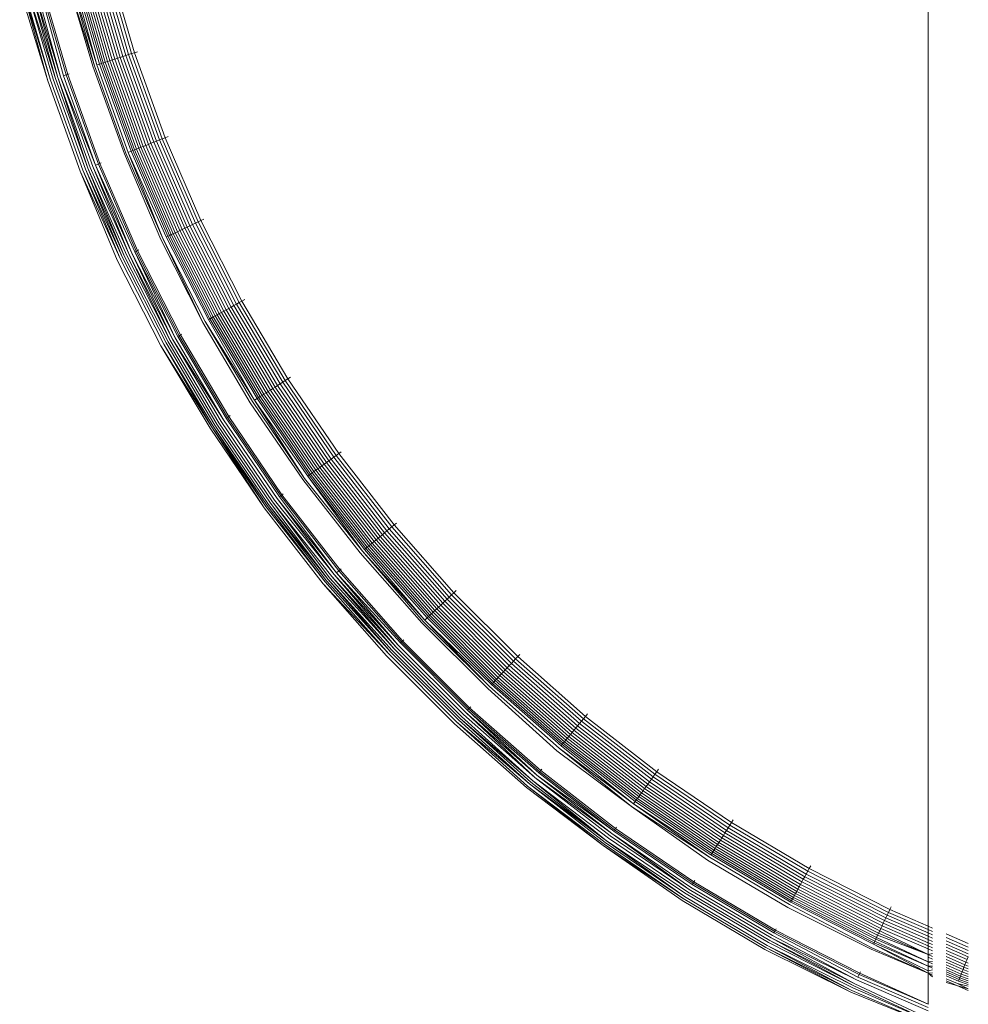
# Model space of a CAD drawing. Units: inches. Extents: x 64 to 1167, y 117 to 939.
# Tile 42 of 56: x 1129.1618 to 1129.8616, y 499.9133 to 500.6393. Entities that reach past the tile are written whole.
import ezdxf

# ---------------------------------------------------------------- set-up
doc = ezdxf.new("R2010")
doc.units = ezdxf.units.IN
doc.header["$MEASUREMENT"] = 0
doc.layers.add('A-FLOR-FIXT', color=8, linetype='Continuous', lineweight=18)

msp = doc.modelspace()

# ---------------------------------------------------------------- linework, layer by layer
at = {"layer": 'A-FLOR-FIXT'}
for p, q in [((1129.83185, 499.97088), (1129.83185, 500.69852)), ((1129.20936, 500.67419), (1129.22829, 500.60906)), ((1129.21118, 500.67466), (1129.23007, 500.60964)), ((1129.21308, 500.67515), (1129.23194, 500.61024)), ((1129.21505, 500.67566), (1129.23387, 500.61087)), ((1129.21709, 500.67618), (1129.23587, 500.61152)), ((1129.21918, 500.67672), (1129.23793, 500.61219)), ((1129.22132, 500.67727), (1129.24003, 500.61288)), ((1129.2235, 500.67783), (1129.24217, 500.61357)), ((1129.22571, 500.67839), (1129.24434, 500.61427)), ((1129.22794, 500.67896), (1129.24652, 500.61498)), ((1129.19606, 500.67078), (1129.21694, 500.60537)), ((1129.19606, 500.67078), (1129.2158, 500.605)), ((1129.19859, 500.67143), (1129.21862, 500.60592)), ((1129.19859, 500.67143), (1129.21694, 500.60537)), ((1129.20057, 500.67194), (1129.21862, 500.60592)), ((1129.20175, 500.67224), (1129.22081, 500.60663)), ((1129.20305, 500.67257), (1129.22209, 500.60705)), ((1129.20447, 500.67294), (1129.22348, 500.6075)), ((1129.206, 500.67333), (1129.22498, 500.60799)), ((1129.20763, 500.67375), (1129.22659, 500.60851)), ((1129.16182, 500.66199), (1129.1825, 500.59418)), ((1129.16358, 500.66244), (1129.1825, 500.59418)), ((1129.16358, 500.66244), (1129.18443, 500.59481)), ((1129.1647, 500.66273), (1129.18443, 500.59481)), ((1129.16683, 500.66327), (1129.18817, 500.59602)), ((1129.16683, 500.66327), (1129.18652, 500.59549)), ((1129.16942, 500.66394), (1129.19, 500.59662)), ((1129.16942, 500.66394), (1129.18817, 500.59602)), ((1129.17135, 500.66444), (1129.19197, 500.59726)), ((1129.17135, 500.66444), (1129.19, 500.59662)), ((1129.17342, 500.66497), (1129.19197, 500.59726)), ((1129.17558, 500.66552), (1129.19404, 500.59793)), ((1129.17668, 500.6658), (1129.1962, 500.59863)), ((1129.1778, 500.66609), (1129.19729, 500.59899)), ((1129.22829, 500.60906), (1129.22659, 500.60851)), ((1129.23007, 500.60964), (1129.22829, 500.60906)), ((1129.22829, 500.60906), (1129.25126, 500.54524)), ((1129.23194, 500.61024), (1129.23007, 500.60964)), ((1129.23007, 500.60964), (1129.25301, 500.54593)), ((1129.23387, 500.61087), (1129.23194, 500.61024)), ((1129.23194, 500.61024), (1129.25483, 500.54665)), ((1129.23587, 500.61152), (1129.23387, 500.61087)), ((1129.23387, 500.61087), (1129.25672, 500.5474)), ((1129.23793, 500.61219), (1129.23587, 500.61152)), ((1129.23587, 500.61152), (1129.25868, 500.54818)), ((1129.24003, 500.61288), (1129.23793, 500.61219)), ((1129.23793, 500.61219), (1129.26069, 500.54897)), ((1129.24217, 500.61357), (1129.24003, 500.61288)), ((1129.24003, 500.61288), (1129.26274, 500.54979)), ((1129.24434, 500.61427), (1129.24217, 500.61357)), ((1129.24217, 500.61357), (1129.26484, 500.55061)), ((1129.24652, 500.61498), (1129.24434, 500.61427)), ((1129.24434, 500.61427), (1129.26695, 500.55145)), ((1129.24872, 500.6157), (1129.24652, 500.61498)), ((1129.24652, 500.61498), (1129.26909, 500.5523)), ((1129.2158, 500.605), (1129.23905, 500.54041)), ((1129.21694, 500.60537), (1129.24017, 500.54085)), ((1129.22081, 500.60663), (1129.21862, 500.60592)), ((1129.21862, 500.60592), (1129.24181, 500.5415)), ((1129.22209, 500.60705), (1129.22081, 500.60663)), ((1129.22081, 500.60663), (1129.24395, 500.54235)), ((1129.22348, 500.6075), (1129.22209, 500.60705)), ((1129.22209, 500.60705), (1129.2452, 500.54284)), ((1129.22498, 500.60799), (1129.22348, 500.6075)), ((1129.22348, 500.6075), (1129.24657, 500.54338)), ((1129.22659, 500.60851), (1129.22498, 500.60799)), ((1129.22498, 500.60799), (1129.24803, 500.54396)), ((1129.22659, 500.60851), (1129.2496, 500.54458)), ((1129.18443, 500.59481), (1129.20839, 500.52827)), ((1129.18652, 500.59549), (1129.21043, 500.52907)), ((1129.18817, 500.59602), (1129.21205, 500.52971)), ((1129.19, 500.59662), (1129.21383, 500.53042)), ((1129.19, 500.59662), (1129.21205, 500.52971)), ((1129.19197, 500.59726), (1129.21575, 500.53118)), ((1129.19197, 500.59726), (1129.21779, 500.53199)), ((1129.1962, 500.59863), (1129.19404, 500.59793)), ((1129.19404, 500.59793), (1129.21779, 500.53199)), ((1129.19729, 500.59899), (1129.1962, 500.59863)), ((1129.1962, 500.59863), (1129.21989, 500.53282)), ((1129.19839, 500.59934), (1129.19729, 500.59899)), ((1129.19729, 500.59899), (1129.22096, 500.53324)), ((1129.1825, 500.59418), (1129.2065, 500.52752)), ((1129.26695, 500.55145), (1129.26484, 500.55061)), ((1129.26909, 500.5523), (1129.26695, 500.55145)), ((1129.26695, 500.55145), (1129.29347, 500.49018)), ((1129.27124, 500.55315), (1129.26909, 500.5523)), ((1129.26909, 500.5523), (1129.29555, 500.49115)), ((1129.2452, 500.54284), (1129.24657, 500.54338)), ((1129.24657, 500.54338), (1129.24803, 500.54396)), ((1129.24657, 500.54338), (1129.27363, 500.48084)), ((1129.24803, 500.54396), (1129.2496, 500.54458)), ((1129.24803, 500.54396), (1129.27506, 500.48151)), ((1129.2496, 500.54458), (1129.25126, 500.54524)), ((1129.2496, 500.54458), (1129.27658, 500.48223)), ((1129.25126, 500.54524), (1129.25301, 500.54593)), ((1129.25126, 500.54524), (1129.2782, 500.48299)), ((1129.25483, 500.54665), (1129.25301, 500.54593)), ((1129.25301, 500.54593), (1129.2799, 500.48379)), ((1129.25672, 500.5474), (1129.25483, 500.54665)), ((1129.25483, 500.54665), (1129.28167, 500.48462)), ((1129.25868, 500.54818), (1129.25672, 500.5474)), ((1129.25672, 500.5474), (1129.28352, 500.48549)), ((1129.26069, 500.54897), (1129.25868, 500.54818)), ((1129.25868, 500.54818), (1129.28542, 500.48639)), ((1129.26274, 500.54979), (1129.26069, 500.54897)), ((1129.26069, 500.54897), (1129.28738, 500.48731)), ((1129.26484, 500.55061), (1129.26274, 500.54979)), ((1129.26274, 500.54979), (1129.28937, 500.48825)), ((1129.26484, 500.55061), (1129.29141, 500.48921)), ((1129.23905, 500.54041), (1129.26598, 500.47724)), ((1129.24017, 500.54085), (1129.2674, 500.47791)), ((1129.24181, 500.5415), (1129.24395, 500.54235)), ((1129.24181, 500.5415), (1129.26998, 500.47912)), ((1129.24181, 500.5415), (1129.2674, 500.47791)), ((1129.24395, 500.54235), (1129.2452, 500.54284)), ((1129.24395, 500.54235), (1129.27109, 500.47964)), ((1129.2452, 500.54284), (1129.27231, 500.48022)), ((1129.21043, 500.52907), (1129.23775, 500.46396)), ((1129.21043, 500.52907), (1129.23923, 500.46465)), ((1129.21205, 500.52971), (1129.24089, 500.46543)), ((1129.21205, 500.52971), (1129.23923, 500.46465)), ((1129.21383, 500.53042), (1129.24269, 500.46628)), ((1129.21575, 500.53118), (1129.24269, 500.46628)), ((1129.21575, 500.53118), (1129.24462, 500.46719)), ((1129.21989, 500.53282), (1129.21779, 500.53199)), ((1129.21779, 500.53199), (1129.24664, 500.46814)), ((1129.21779, 500.53199), (1129.24462, 500.46719)), ((1129.22096, 500.53324), (1129.21989, 500.53282)), ((1129.21989, 500.53282), (1129.24767, 500.46862)), ((1129.22203, 500.53367), (1129.22096, 500.53324)), ((1129.22096, 500.53324), (1129.24871, 500.46911)), ((1129.2065, 500.52752), (1129.23382, 500.46211)), ((1129.2065, 500.52752), (1129.23593, 500.4631)), ((1129.20839, 500.52827), (1129.23593, 500.4631)), ((1129.20839, 500.52827), (1129.23775, 500.46396)), ((1129.28352, 500.48549), (1129.28167, 500.48462)), ((1129.28542, 500.48639), (1129.28352, 500.48549)), ((1129.28352, 500.48549), (1129.31414, 500.42538)), ((1129.28738, 500.48731), (1129.28542, 500.48639)), ((1129.28542, 500.48639), (1129.31599, 500.4264)), ((1129.28937, 500.48825), (1129.28738, 500.48731)), ((1129.28738, 500.48731), (1129.31788, 500.42744)), ((1129.29141, 500.48921), (1129.28937, 500.48825)), ((1129.28937, 500.48825), (1129.31982, 500.4285)), ((1129.29347, 500.49018), (1129.29141, 500.48921)), ((1129.29141, 500.48921), (1129.32179, 500.42959)), ((1129.29555, 500.49115), (1129.29347, 500.49018)), ((1129.29347, 500.49018), (1129.32378, 500.43068)), ((1129.29764, 500.49214), (1129.29555, 500.49115)), ((1129.29555, 500.49115), (1129.3258, 500.43179)), ((1129.27109, 500.47964), (1129.26998, 500.47912)), ((1129.26998, 500.47912), (1129.30104, 500.41818)), ((1129.27231, 500.48022), (1129.27109, 500.47964)), ((1129.27109, 500.47964), (1129.30211, 500.41877)), ((1129.27363, 500.48084), (1129.27231, 500.48022)), ((1129.27231, 500.48022), (1129.30328, 500.41941)), ((1129.27506, 500.48151), (1129.27363, 500.48084)), ((1129.27363, 500.48084), (1129.30457, 500.42012)), ((1129.27658, 500.48223), (1129.27506, 500.48151)), ((1129.27506, 500.48151), (1129.30595, 500.42088)), ((1129.2782, 500.48299), (1129.27658, 500.48223)), ((1129.27658, 500.48223), (1129.30743, 500.42169)), ((1129.2799, 500.48379), (1129.2782, 500.48299)), ((1129.2782, 500.48299), (1129.30899, 500.42255)), ((1129.28167, 500.48462), (1129.2799, 500.48379)), ((1129.2799, 500.48379), (1129.31064, 500.42346)), ((1129.28167, 500.48462), (1129.31236, 500.4244)), ((1129.26598, 500.47724), (1129.29696, 500.41594)), ((1129.2674, 500.47791), (1129.29854, 500.4168)), ((1129.2674, 500.47791), (1129.29696, 500.41594)), ((1129.23775, 500.46396), (1129.26982, 500.40102)), ((1129.23923, 500.46465), (1129.27125, 500.4018)), ((1129.24089, 500.46543), (1129.27285, 500.40269)), ((1129.24269, 500.46628), (1129.27461, 500.40365)), ((1129.24269, 500.46628), (1129.27285, 500.40269)), ((1129.24462, 500.46719), (1129.27648, 500.40468)), ((1129.24462, 500.46719), (1129.27461, 500.40365)), ((1129.24664, 500.46814), (1129.24767, 500.46862)), ((1129.24664, 500.46814), (1129.27843, 500.40575)), ((1129.24664, 500.46814), (1129.27648, 500.40468)), ((1129.24767, 500.46862), (1129.24871, 500.46911)), ((1129.24767, 500.46862), (1129.27943, 500.4063)), ((1129.24871, 500.46911), (1129.24976, 500.4696)), ((1129.24871, 500.46911), (1129.28043, 500.40685)), ((1129.23382, 500.46211), (1129.26602, 500.39893)), ((1129.23593, 500.4631), (1129.26805, 500.40005)), ((1129.31788, 500.42744), (1129.31599, 500.4264)), ((1129.31982, 500.4285), (1129.31788, 500.42744)), ((1129.31788, 500.42744), (1129.35208, 500.3696)), ((1129.32179, 500.42959), (1129.31982, 500.4285)), ((1129.31982, 500.4285), (1129.35395, 500.37079)), ((1129.32378, 500.43068), (1129.32179, 500.42959)), ((1129.32179, 500.42959), (1129.35585, 500.37199)), ((1129.3258, 500.43179), (1129.32378, 500.43068)), ((1129.32378, 500.43068), (1129.35777, 500.37321)), ((1129.32782, 500.4329), (1129.3258, 500.43179)), ((1129.3258, 500.43179), (1129.35971, 500.37445)), ((1129.30457, 500.42012), (1129.30328, 500.41941)), ((1129.30595, 500.42088), (1129.30457, 500.42012)), ((1129.30457, 500.42012), (1129.33926, 500.36146)), ((1129.30743, 500.42169), (1129.30595, 500.42088)), ((1129.30595, 500.42088), (1129.34059, 500.36231)), ((1129.30899, 500.42255), (1129.30743, 500.42169)), ((1129.30743, 500.42169), (1129.34201, 500.36321)), ((1129.31064, 500.42346), (1129.30899, 500.42255)), ((1129.30899, 500.42255), (1129.34352, 500.36417)), ((1129.31236, 500.4244), (1129.31064, 500.42346)), ((1129.31064, 500.42346), (1129.34511, 500.36518)), ((1129.31414, 500.42538), (1129.31236, 500.4244)), ((1129.31236, 500.4244), (1129.34676, 500.36623)), ((1129.31599, 500.4264), (1129.31414, 500.42538)), ((1129.31414, 500.42538), (1129.34848, 500.36732)), ((1129.31599, 500.4264), (1129.35026, 500.36845)), ((1129.29696, 500.41594), (1129.33193, 500.35681)), ((1129.29854, 500.4168), (1129.33494, 500.35872)), ((1129.29854, 500.4168), (1129.33344, 500.35778)), ((1129.30211, 500.41877), (1129.30104, 500.41818)), ((1129.30104, 500.41818), (1129.33494, 500.35872)), ((1129.30328, 500.41941), (1129.30211, 500.41877)), ((1129.30211, 500.41877), (1129.33689, 500.35996)), ((1129.30328, 500.41941), (1129.33802, 500.36068)), ((1129.27943, 500.4063), (1129.27843, 500.40575)), ((1129.27843, 500.40575), (1129.31407, 500.34548)), ((1129.28043, 500.40685), (1129.27943, 500.4063)), ((1129.27943, 500.4063), (1129.31503, 500.34609)), ((1129.28145, 500.40741), (1129.28043, 500.40685)), ((1129.28043, 500.40685), (1129.316, 500.34671)), ((1129.26602, 500.39893), (1129.30237, 500.33805)), ((1129.26602, 500.39893), (1129.30362, 500.33885)), ((1129.26805, 500.40005), (1129.30459, 500.33946)), ((1129.26805, 500.40005), (1129.30362, 500.33885)), ((1129.26982, 500.40102), (1129.30578, 500.34022)), ((1129.27125, 500.4018), (1129.30716, 500.34109)), ((1129.27285, 500.40269), (1129.3087, 500.34207)), ((1129.27461, 500.40365), (1129.31039, 500.34314)), ((1129.27461, 500.40365), (1129.31219, 500.34429)), ((1129.27648, 500.40468), (1129.31219, 500.34429)), ((1129.35208, 500.3696), (1129.35026, 500.36845)), ((1129.35395, 500.37079), (1129.35208, 500.3696)), ((1129.35208, 500.3696), (1129.38985, 500.31403)), ((1129.35585, 500.37199), (1129.35395, 500.37079)), ((1129.35395, 500.37079), (1129.39164, 500.31533)), ((1129.35777, 500.37321), (1129.35585, 500.37199)), ((1129.35585, 500.37199), (1129.39346, 500.31665)), ((1129.35971, 500.37445), (1129.35777, 500.37321)), ((1129.35777, 500.37321), (1129.3953, 500.31799)), ((1129.36166, 500.37568), (1129.35971, 500.37445)), ((1129.35971, 500.37445), (1129.39716, 500.31934)), ((1129.33926, 500.36146), (1129.34059, 500.36231)), ((1129.34059, 500.36231), (1129.34201, 500.36321)), ((1129.34059, 500.36231), (1129.37884, 500.30603)), ((1129.34201, 500.36321), (1129.34352, 500.36417)), ((1129.34201, 500.36321), (1129.3802, 500.30702)), ((1129.34352, 500.36417), (1129.34511, 500.36518)), ((1129.34352, 500.36417), (1129.38165, 500.30807)), ((1129.34511, 500.36518), (1129.34676, 500.36623)), ((1129.34511, 500.36518), (1129.38317, 500.30917)), ((1129.34848, 500.36732), (1129.34676, 500.36623)), ((1129.34676, 500.36623), (1129.38475, 500.31033)), ((1129.35026, 500.36845), (1129.34848, 500.36732)), ((1129.34848, 500.36732), (1129.3864, 500.31152)), ((1129.35026, 500.36845), (1129.3881, 500.31276)), ((1129.33193, 500.35681), (1129.37072, 500.30013)), ((1129.33344, 500.35778), (1129.37199, 500.30105)), ((1129.33494, 500.35872), (1129.33689, 500.35996)), ((1129.33494, 500.35872), (1129.3743, 500.30273)), ((1129.33494, 500.35872), (1129.37199, 500.30105)), ((1129.33689, 500.35996), (1129.33802, 500.36068)), ((1129.33689, 500.35996), (1129.37529, 500.30345)), ((1129.33802, 500.36068), (1129.33926, 500.36146)), ((1129.33802, 500.36068), (1129.37638, 500.30424)), ((1129.33926, 500.36146), (1129.37756, 500.3051)), ((1129.316, 500.34671), (1129.31698, 500.34733)), ((1129.30578, 500.34022), (1129.34548, 500.28179)), ((1129.30716, 500.34109), (1129.3468, 500.28275)), ((1129.3087, 500.34207), (1129.34828, 500.28383)), ((1129.31039, 500.34314), (1129.3499, 500.285)), ((1129.31219, 500.34429), (1129.35163, 500.28626)), ((1129.31407, 500.34548), (1129.31503, 500.34609)), ((1129.31407, 500.34548), (1129.35343, 500.28757)), ((1129.31503, 500.34609), (1129.316, 500.34671)), ((1129.31503, 500.34609), (1129.35435, 500.28824)), ((1129.316, 500.34671), (1129.35528, 500.28891)), ((1129.30237, 500.33805), (1129.34221, 500.27942)), ((1129.30362, 500.33885), (1129.34341, 500.28029)), ((1129.30362, 500.33885), (1129.34221, 500.27942)), ((1129.30459, 500.33946), (1129.34434, 500.28097)), ((1129.30459, 500.33946), (1129.34341, 500.28029)), ((1129.3953, 500.31799), (1129.39716, 500.31934)), ((1129.39716, 500.31934), (1129.39903, 500.3207)), ((1129.39716, 500.31934), (1129.438, 500.2667)), ((1129.38475, 500.31033), (1129.3864, 500.31152)), ((1129.3864, 500.31152), (1129.3881, 500.31276)), ((1129.3864, 500.31152), (1129.42775, 500.25822)), ((1129.3881, 500.31276), (1129.38985, 500.31403)), ((1129.3881, 500.31276), (1129.42937, 500.25956)), ((1129.38985, 500.31403), (1129.39164, 500.31533)), ((1129.38985, 500.31403), (1129.43103, 500.26094)), ((1129.39164, 500.31533), (1129.39346, 500.31665)), ((1129.39164, 500.31533), (1129.43274, 500.26235)), ((1129.39346, 500.31665), (1129.3953, 500.31799)), ((1129.39346, 500.31665), (1129.43447, 500.26378)), ((1129.3953, 500.31799), (1129.43622, 500.26523)), ((1129.37638, 500.30424), (1129.37529, 500.30345)), ((1129.37756, 500.3051), (1129.37638, 500.30424)), ((1129.37638, 500.30424), (1129.4182, 500.25032)), ((1129.37884, 500.30603), (1129.37756, 500.3051)), ((1129.37756, 500.3051), (1129.41933, 500.25126)), ((1129.3802, 500.30702), (1129.37884, 500.30603)), ((1129.37884, 500.30603), (1129.42055, 500.25226)), ((1129.38165, 500.30807), (1129.3802, 500.30702)), ((1129.3802, 500.30702), (1129.42184, 500.25334)), ((1129.38317, 500.30917), (1129.38165, 500.30807)), ((1129.38165, 500.30807), (1129.42322, 500.25447)), ((1129.38475, 500.31033), (1129.38317, 500.30917)), ((1129.38317, 500.30917), (1129.42467, 500.25567)), ((1129.38475, 500.31033), (1129.42618, 500.25692)), ((1129.37072, 500.30013), (1129.4131, 500.24611)), ((1129.37199, 500.30105), (1129.41465, 500.24739)), ((1129.37529, 500.30345), (1129.3743, 500.30273)), ((1129.3743, 500.30273), (1129.41465, 500.24739)), ((1129.3743, 500.30273), (1129.41622, 500.24869)), ((1129.37529, 500.30345), (1129.41716, 500.24946)), ((1129.35528, 500.28891), (1129.35621, 500.28959)), ((1129.3468, 500.28275), (1129.38938, 500.22648)), ((1129.34828, 500.28383), (1129.3922, 500.22881)), ((1129.34828, 500.28383), (1129.39072, 500.22759)), ((1129.3499, 500.285), (1129.39379, 500.23013)), ((1129.35163, 500.28626), (1129.39548, 500.23152)), ((1129.35163, 500.28626), (1129.39379, 500.23013)), ((1129.35343, 500.28757), (1129.35435, 500.28824)), ((1129.35343, 500.28757), (1129.39548, 500.23152)), ((1129.35435, 500.28824), (1129.35528, 500.28891)), ((1129.35435, 500.28824), (1129.39722, 500.23297)), ((1129.35528, 500.28891), (1129.39811, 500.2337)), ((1129.34221, 500.27942), (1129.38566, 500.2234)), ((1129.34341, 500.28029), (1129.38722, 500.2247)), ((1129.34434, 500.28097), (1129.38722, 500.2247)), ((1129.34548, 500.28179), (1129.38938, 500.22648)), ((1129.34548, 500.28179), (1129.38821, 500.22551)), ((1129.43977, 500.26817), (1129.438, 500.2667)), ((1129.43103, 500.26094), (1129.42937, 500.25956)), ((1129.43274, 500.26235), (1129.43103, 500.26094)), ((1129.43103, 500.26094), (1129.47547, 500.21054)), ((1129.43447, 500.26378), (1129.43274, 500.26235)), ((1129.43274, 500.26235), (1129.47708, 500.21205)), ((1129.43622, 500.26523), (1129.43447, 500.26378)), ((1129.43447, 500.26378), (1129.47872, 500.21359)), ((1129.438, 500.2667), (1129.43622, 500.26523)), ((1129.43622, 500.26523), (1129.48038, 500.21515)), ((1129.438, 500.2667), (1129.48206, 500.21672)), ((1129.42184, 500.25334), (1129.42055, 500.25226)), ((1129.42322, 500.25447), (1129.42184, 500.25334)), ((1129.42184, 500.25334), (1129.46677, 500.20237)), ((1129.42467, 500.25567), (1129.42322, 500.25447)), ((1129.42322, 500.25447), (1129.46808, 500.2036)), ((1129.42618, 500.25692), (1129.42467, 500.25567)), ((1129.42467, 500.25567), (1129.46944, 500.20488)), ((1129.42775, 500.25822), (1129.42618, 500.25692)), ((1129.42618, 500.25692), (1129.47087, 500.20622)), ((1129.42937, 500.25956), (1129.42775, 500.25822)), ((1129.42775, 500.25822), (1129.47236, 500.20762)), ((1129.42937, 500.25956), (1129.47389, 500.20906)), ((1129.4131, 500.24611), (1129.45851, 500.19461)), ((1129.41465, 500.24739), (1129.46066, 500.19663)), ((1129.41465, 500.24739), (1129.45938, 500.19543)), ((1129.41716, 500.24946), (1129.41622, 500.24869)), ((1129.41622, 500.24869), (1129.46066, 500.19663)), ((1129.4182, 500.25032), (1129.41716, 500.24946)), ((1129.41716, 500.24946), (1129.46235, 500.19821)), ((1129.41933, 500.25126), (1129.4182, 500.25032)), ((1129.4182, 500.25032), (1129.46333, 500.19914)), ((1129.42055, 500.25226), (1129.41933, 500.25126)), ((1129.41933, 500.25126), (1129.4644, 500.20014)), ((1129.42055, 500.25226), (1129.46555, 500.20122)), ((1129.39722, 500.23297), (1129.39548, 500.23152)), ((1129.39548, 500.23152), (1129.44265, 500.17972)), ((1129.39548, 500.23152), (1129.44103, 500.17819)), ((1129.39811, 500.2337), (1129.39722, 500.23297)), ((1129.39722, 500.23297), (1129.44348, 500.1805)), ((1129.399, 500.23444), (1129.39811, 500.2337)), ((1129.39811, 500.2337), (1129.44432, 500.18129)), ((1129.38722, 500.2247), (1129.43402, 500.17161)), ((1129.38821, 500.22551), (1129.43549, 500.17299)), ((1129.38938, 500.22648), (1129.43668, 500.17411)), ((1129.38938, 500.22648), (1129.43549, 500.17299)), ((1129.39072, 500.22759), (1129.43801, 500.17536)), ((1129.3922, 500.22881), (1129.43947, 500.17673)), ((1129.3922, 500.22881), (1129.43801, 500.17536)), ((1129.39379, 500.23013), (1129.44103, 500.17819)), ((1129.39379, 500.23013), (1129.43947, 500.17673)), ((1129.38566, 500.2234), (1129.43241, 500.1701)), ((1129.38566, 500.2234), (1129.43402, 500.17161)), ((1129.48206, 500.21672), (1129.48038, 500.21515)), ((1129.48374, 500.2183), (1129.48206, 500.21672)), ((1129.48206, 500.21672), (1129.52917, 500.16961)), ((1129.47547, 500.21054), (1129.47389, 500.20906)), ((1129.47708, 500.21205), (1129.47547, 500.21054)), ((1129.47547, 500.21054), (1129.52298, 500.16302)), ((1129.47872, 500.21359), (1129.47708, 500.21205)), ((1129.47708, 500.21205), (1129.52449, 500.16464)), ((1129.48038, 500.21515), (1129.47872, 500.21359)), ((1129.47872, 500.21359), (1129.52603, 500.16628)), ((1129.48038, 500.21515), (1129.52759, 500.16794)), ((1129.46677, 500.20237), (1129.46555, 500.20122)), ((1129.46808, 500.2036), (1129.46677, 500.20237)), ((1129.46677, 500.20237), (1129.51482, 500.15433)), ((1129.46944, 500.20488), (1129.46808, 500.2036)), ((1129.46808, 500.2036), (1129.51604, 500.15563)), ((1129.47087, 500.20622), (1129.46944, 500.20488)), ((1129.46944, 500.20488), (1129.51732, 500.157)), ((1129.47236, 500.20762), (1129.47087, 500.20622)), ((1129.47087, 500.20622), (1129.51867, 500.15843)), ((1129.47389, 500.20906), (1129.47236, 500.20762)), ((1129.47236, 500.20762), (1129.52006, 500.15992)), ((1129.47389, 500.20906), (1129.5215, 500.16145)), ((1129.45938, 500.19543), (1129.50843, 500.14753)), ((1129.46235, 500.19821), (1129.46066, 500.19663)), ((1129.46066, 500.19663), (1129.50843, 500.14753)), ((1129.46066, 500.19663), (1129.50982, 500.14901)), ((1129.46333, 500.19914), (1129.46235, 500.19821)), ((1129.46235, 500.19821), (1129.51066, 500.1499)), ((1129.4644, 500.20014), (1129.46333, 500.19914)), ((1129.46333, 500.19914), (1129.51158, 500.15088)), ((1129.46555, 500.20122), (1129.4644, 500.20014)), ((1129.4644, 500.20014), (1129.51258, 500.15195)), ((1129.46555, 500.20122), (1129.51366, 500.1531)), ((1129.45851, 500.19461), (1129.50705, 500.14606)), ((1129.44265, 500.17972), (1129.44348, 500.1805)), ((1129.44348, 500.1805), (1129.44432, 500.18129)), ((1129.44348, 500.1805), (1129.49294, 500.13104)), ((1129.44432, 500.18129), (1129.44516, 500.18208)), ((1129.44432, 500.18129), (1129.49373, 500.13188)), ((1129.43668, 500.17411), (1129.48655, 500.12424)), ((1129.43801, 500.17536), (1129.48781, 500.12557)), ((1129.43947, 500.17673), (1129.48918, 500.12703)), ((1129.44103, 500.17819), (1129.49064, 500.12858)), ((1129.44265, 500.17972), (1129.49216, 500.13021)), ((1129.43241, 500.1701), (1129.48254, 500.11996)), ((1129.43402, 500.17161), (1129.48406, 500.12158)), ((1129.43549, 500.17299), (1129.48544, 500.12305)), ((1129.52603, 500.16628), (1129.52449, 500.16464)), ((1129.52759, 500.16794), (1129.52603, 500.16628)), ((1129.52603, 500.16628), (1129.57622, 500.12203)), ((1129.52917, 500.16961), (1129.52759, 500.16794)), ((1129.52759, 500.16794), (1129.57768, 500.12378)), ((1129.53075, 500.17129), (1129.52917, 500.16961)), ((1129.52917, 500.16961), (1129.57914, 500.12555)), ((1129.52006, 500.15992), (1129.51867, 500.15843)), ((1129.5215, 500.16145), (1129.52006, 500.15992)), ((1129.52006, 500.15992), (1129.57066, 500.1153)), ((1129.52298, 500.16302), (1129.5215, 500.16145)), ((1129.5215, 500.16145), (1129.572, 500.11692)), ((1129.52449, 500.16464), (1129.52298, 500.16302)), ((1129.52298, 500.16302), (1129.57338, 500.11859)), ((1129.52449, 500.16464), (1129.57479, 500.12029)), ((1129.51258, 500.15195), (1129.51158, 500.15088)), ((1129.51366, 500.1531), (1129.51258, 500.15195)), ((1129.51258, 500.15195), (1129.5637, 500.10689)), ((1129.51482, 500.15433), (1129.51366, 500.1531)), ((1129.51366, 500.1531), (1129.56471, 500.1081)), ((1129.51604, 500.15563), (1129.51482, 500.15433)), ((1129.51482, 500.15433), (1129.56578, 500.1094)), ((1129.51732, 500.157), (1129.51604, 500.15563)), ((1129.51604, 500.15563), (1129.56692, 500.11078)), ((1129.51867, 500.15843), (1129.51732, 500.157)), ((1129.51732, 500.157), (1129.56811, 500.11222)), ((1129.51867, 500.15843), (1129.56936, 500.11373)), ((1129.50705, 500.14606), (1129.55816, 500.1002)), ((1129.50843, 500.14753), (1129.55983, 500.10221)), ((1129.51066, 500.1499), (1129.50982, 500.14901)), ((1129.50982, 500.14901), (1129.56113, 500.10378)), ((1129.51158, 500.15088), (1129.51066, 500.1499)), ((1129.51066, 500.1499), (1129.56191, 500.10472)), ((1129.51158, 500.15088), (1129.56277, 500.10576)), ((1129.49216, 500.13021), (1129.49294, 500.13104)), ((1129.49216, 500.13021), (1129.54326, 500.08218)), ((1129.49216, 500.13021), (1129.54469, 500.0839)), ((1129.49294, 500.13104), (1129.49373, 500.13188)), ((1129.49294, 500.13104), (1129.54541, 500.08478)), ((1129.49373, 500.13188), (1129.49452, 500.13272)), ((1129.49373, 500.13188), (1129.54614, 500.08567)), ((1129.48544, 500.12305), (1129.53796, 500.07577)), ((1129.48655, 500.12424), (1129.54003, 500.07828)), ((1129.48655, 500.12424), (1129.53893, 500.07694)), ((1129.48781, 500.12557), (1129.54003, 500.07828)), ((1129.48918, 500.12703), (1129.5419, 500.08054)), ((1129.49064, 500.12858), (1129.54326, 500.08218)), ((1129.49064, 500.12858), (1129.5419, 500.08054)), ((1129.57768, 500.12378), (1129.57622, 500.12203)), ((1129.57914, 500.12555), (1129.57768, 500.12378)), ((1129.57768, 500.12378), (1129.63043, 500.08286)), ((1129.58061, 500.12733), (1129.57914, 500.12555)), ((1129.57914, 500.12555), (1129.63178, 500.08472)), ((1129.48254, 500.11996), (1129.53573, 500.07307)), ((1129.48406, 500.12158), (1129.53649, 500.07399)), ((1129.48406, 500.12158), (1129.53796, 500.07577)), ((1129.57066, 500.1153), (1129.56936, 500.11373)), ((1129.572, 500.11692), (1129.57066, 500.1153)), ((1129.57066, 500.1153), (1129.62397, 500.07396)), ((1129.57338, 500.11859), (1129.572, 500.11692)), ((1129.572, 500.11692), (1129.6252, 500.07566)), ((1129.57479, 500.12029), (1129.57338, 500.11859)), ((1129.57338, 500.11859), (1129.62647, 500.07741)), ((1129.57622, 500.12203), (1129.57479, 500.12029)), ((1129.57479, 500.12029), (1129.62777, 500.0792)), ((1129.57622, 500.12203), (1129.62909, 500.08101)), ((1129.56471, 500.1081), (1129.5637, 500.10689)), ((1129.56578, 500.1094), (1129.56471, 500.1081)), ((1129.56471, 500.1081), (1129.61847, 500.0664)), ((1129.56692, 500.11078), (1129.56578, 500.1094)), ((1129.56578, 500.1094), (1129.61946, 500.06776)), ((1129.56811, 500.11222), (1129.56692, 500.11078)), ((1129.56692, 500.11078), (1129.62051, 500.0692)), ((1129.56936, 500.11373), (1129.56811, 500.11222)), ((1129.56811, 500.11222), (1129.62162, 500.07072)), ((1129.56936, 500.11373), (1129.62277, 500.07231)), ((1129.55983, 500.10221), (1129.61454, 500.06098)), ((1129.55983, 500.10221), (1129.6131, 500.05901)), ((1129.56191, 500.10472), (1129.56113, 500.10378)), ((1129.56113, 500.10378), (1129.61454, 500.06098)), ((1129.56277, 500.10576), (1129.56191, 500.10472)), ((1129.56191, 500.10472), (1129.61589, 500.06284)), ((1129.5637, 500.10689), (1129.56277, 500.10576)), ((1129.56277, 500.10576), (1129.61668, 500.06393)), ((1129.5637, 500.10689), (1129.61755, 500.06512)), ((1129.55816, 500.1002), (1129.6131, 500.05901)), ((1129.54688, 500.08655), (1129.54614, 500.08567)), ((1129.63314, 500.08659), (1129.63178, 500.08472)), ((1129.5419, 500.08054), (1129.59745, 500.03746)), ((1129.5419, 500.08054), (1129.5987, 500.03918)), ((1129.54326, 500.08218), (1129.5987, 500.03918)), ((1129.54326, 500.08218), (1129.60001, 500.04099)), ((1129.54541, 500.08478), (1129.54469, 500.0839)), ((1129.54469, 500.0839), (1129.60001, 500.04099)), ((1129.54614, 500.08567), (1129.54541, 500.08478)), ((1129.54541, 500.08478), (1129.60068, 500.04191)), ((1129.54614, 500.08567), (1129.60136, 500.04284)), ((1129.62777, 500.0792), (1129.62647, 500.07741)), ((1129.62909, 500.08101), (1129.62777, 500.0792)), ((1129.62777, 500.0792), (1129.68323, 500.04151)), ((1129.63043, 500.08286), (1129.62909, 500.08101)), ((1129.62909, 500.08101), (1129.68444, 500.0434)), ((1129.63178, 500.08472), (1129.63043, 500.08286)), ((1129.63043, 500.08286), (1129.68566, 500.04533)), ((1129.63178, 500.08472), (1129.68689, 500.04727)), ((1129.53573, 500.07307), (1129.59221, 500.03025)), ((1129.53649, 500.07399), (1129.59305, 500.03141)), ((1129.53649, 500.07399), (1129.59221, 500.03025)), ((1129.53796, 500.07577), (1129.59381, 500.03245)), ((1129.53796, 500.07577), (1129.5947, 500.03368)), ((1129.53893, 500.07694), (1129.5947, 500.03368)), ((1129.54003, 500.07828), (1129.59627, 500.03584)), ((1129.54003, 500.07828), (1129.5947, 500.03368)), ((1129.62162, 500.07072), (1129.62277, 500.07231)), ((1129.62397, 500.07396), (1129.62277, 500.07231)), ((1129.62277, 500.07231), (1129.67867, 500.03432)), ((1129.6252, 500.07566), (1129.62397, 500.07396)), ((1129.62397, 500.07396), (1129.67976, 500.03604)), ((1129.62647, 500.07741), (1129.6252, 500.07566)), ((1129.6252, 500.07566), (1129.68089, 500.03781)), ((1129.62647, 500.07741), (1129.68205, 500.03964)), ((1129.61668, 500.06393), (1129.61755, 500.06512)), ((1129.61755, 500.06512), (1129.61847, 500.0664)), ((1129.61755, 500.06512), (1129.67391, 500.02681)), ((1129.61847, 500.0664), (1129.61946, 500.06776)), ((1129.61847, 500.0664), (1129.67475, 500.02815)), ((1129.61946, 500.06776), (1129.62051, 500.0692)), ((1129.61946, 500.06776), (1129.67566, 500.02957)), ((1129.62051, 500.0692), (1129.62162, 500.07072)), ((1129.62051, 500.0692), (1129.67661, 500.03108)), ((1129.62162, 500.07072), (1129.67762, 500.03266)), ((1129.6131, 500.05901), (1129.66926, 500.01948)), ((1129.6131, 500.05901), (1129.67065, 500.02169)), ((1129.61454, 500.06098), (1129.61589, 500.06284)), ((1129.61454, 500.06098), (1129.67175, 500.02341)), ((1129.61454, 500.06098), (1129.67065, 500.02169)), ((1129.61589, 500.06284), (1129.61668, 500.06393)), ((1129.61589, 500.06284), (1129.6724, 500.02444)), ((1129.61668, 500.06393), (1129.67312, 500.02558)), ((1129.60068, 500.04191), (1129.60136, 500.04284)), ((1129.60136, 500.04284), (1129.60204, 500.04377)), ((1129.60136, 500.04284), (1129.65915, 500.00356)), ((1129.68323, 500.04151), (1129.68444, 500.0434)), ((1129.68444, 500.0434), (1129.68566, 500.04533)), ((1129.68444, 500.0434), (1129.74203, 500.00934)), ((1129.68566, 500.04533), (1129.68689, 500.04727)), ((1129.68566, 500.04533), (1129.74313, 500.01134)), ((1129.68689, 500.04727), (1129.68813, 500.04922)), ((1129.68689, 500.04727), (1129.74423, 500.01335)), ((1129.59627, 500.03584), (1129.65452, 499.99626)), ((1129.59745, 500.03746), (1129.65559, 499.99795)), ((1129.5987, 500.03918), (1129.65673, 499.99975)), ((1129.5987, 500.03918), (1129.65559, 499.99795)), ((1129.60001, 500.04099), (1129.60068, 500.04191)), ((1129.60001, 500.04099), (1129.65792, 500.00163)), ((1129.60068, 500.04191), (1129.65853, 500.00259)), ((1129.67867, 500.03432), (1129.67976, 500.03604)), ((1129.67976, 500.03604), (1129.68089, 500.03781)), ((1129.67976, 500.03604), (1129.73783, 500.0017)), ((1129.68089, 500.03781), (1129.68205, 500.03964)), ((1129.68089, 500.03781), (1129.73884, 500.00354)), ((1129.68205, 500.03964), (1129.68323, 500.04151)), ((1129.68205, 500.03964), (1129.73988, 500.00544)), ((1129.68323, 500.04151), (1129.74095, 500.00737)), ((1129.59221, 500.03025), (1129.65129, 499.99117)), ((1129.59221, 500.03025), (1129.65039, 499.98976)), ((1129.59305, 500.03141), (1129.65129, 499.99117)), ((1129.59381, 500.03245), (1129.65227, 499.99272)), ((1129.5947, 500.03368), (1129.65353, 499.99471)), ((1129.5947, 500.03368), (1129.65227, 499.99272)), ((1129.67391, 500.02681), (1129.67475, 500.02815)), ((1129.67475, 500.02815), (1129.67566, 500.02957)), ((1129.67475, 500.02815), (1129.73332, 499.99351)), ((1129.67566, 500.02957), (1129.67661, 500.03108)), ((1129.67566, 500.02957), (1129.73414, 499.99499)), ((1129.67661, 500.03108), (1129.67762, 500.03266)), ((1129.67661, 500.03108), (1129.735, 499.99655)), ((1129.67762, 500.03266), (1129.67867, 500.03432)), ((1129.67762, 500.03266), (1129.7359, 499.9982)), ((1129.67867, 500.03432), (1129.73685, 499.99991)), ((1129.67065, 500.02169), (1129.72964, 499.9868)), ((1129.67175, 500.02341), (1129.6724, 500.02444)), ((1129.67175, 500.02341), (1129.73062, 499.98859)), ((1129.6724, 500.02444), (1129.67312, 500.02558)), ((1129.6724, 500.02444), (1129.73121, 499.98966)), ((1129.67312, 500.02558), (1129.67391, 500.02681)), ((1129.67312, 500.02558), (1129.73186, 499.99084)), ((1129.67391, 500.02681), (1129.73256, 499.99213)), ((1129.66926, 500.01948), (1129.72849, 499.98472)), ((1129.74313, 500.01134), (1129.74423, 500.01335)), ((1129.74423, 500.01335), (1129.74535, 500.01538)), ((1129.74423, 500.01335), (1129.8036, 499.98311)), ((1129.73988, 500.00544), (1129.74095, 500.00737)), ((1129.74095, 500.00737), (1129.74203, 500.00934)), ((1129.74095, 500.00737), (1129.80069, 499.97693)), ((1129.74203, 500.00934), (1129.74313, 500.01134)), ((1129.74203, 500.00934), (1129.80165, 499.97897)), ((1129.74313, 500.01134), (1129.80262, 499.98103)), ((1129.65673, 499.99975), (1129.71712, 499.96403)), ((1129.65853, 500.00259), (1129.65792, 500.00163)), ((1129.65792, 500.00163), (1129.71819, 499.96599)), ((1129.65915, 500.00356), (1129.65853, 500.00259)), ((1129.65853, 500.00259), (1129.71874, 499.96698)), ((1129.65977, 500.00454), (1129.65915, 500.00356)), ((1129.65915, 500.00356), (1129.7193, 499.96799)), ((1129.7359, 499.9982), (1129.73685, 499.99991)), ((1129.73685, 499.99991), (1129.73783, 500.0017)), ((1129.73685, 499.99991), (1129.79707, 499.96923)), ((1129.73783, 500.0017), (1129.73884, 500.00354)), ((1129.73783, 500.0017), (1129.79793, 499.97107)), ((1129.73884, 500.00354), (1129.73988, 500.00544)), ((1129.73884, 500.00354), (1129.79883, 499.97298)), ((1129.73988, 500.00544), (1129.79975, 499.97493)), ((1129.65227, 499.99272), (1129.71311, 499.95673)), ((1129.65353, 499.99471), (1129.71425, 499.95881)), ((1129.65452, 499.99626), (1129.71513, 499.96041)), ((1129.65559, 499.99795), (1129.71609, 499.96216)), ((1129.73186, 499.99084), (1129.73256, 499.99213)), ((1129.73256, 499.99213), (1129.73332, 499.99351)), ((1129.73256, 499.99213), (1129.79328, 499.96119)), ((1129.73332, 499.99351), (1129.73414, 499.99499)), ((1129.73332, 499.99351), (1129.79396, 499.96262)), ((1129.73414, 499.99499), (1129.735, 499.99655)), ((1129.73414, 499.99499), (1129.79467, 499.96414)), ((1129.735, 499.99655), (1129.7359, 499.9982)), ((1129.735, 499.99655), (1129.79543, 499.96576)), ((1129.7359, 499.9982), (1129.79623, 499.96746)), ((1129.65039, 499.98976), (1129.71142, 499.95367)), ((1129.65129, 499.99117), (1129.71223, 499.95513)), ((1129.72849, 499.98472), (1129.78984, 499.95388)), ((1129.72964, 499.9868), (1129.79035, 499.95496)), ((1129.73121, 499.98966), (1129.73062, 499.98859)), ((1129.73062, 499.98859), (1129.79157, 499.95754)), ((1129.73121, 499.98966), (1129.73186, 499.99084)), ((1129.73121, 499.98966), (1129.79209, 499.95864)), ((1129.73186, 499.99084), (1129.79266, 499.95986)), ((1129.80458, 499.9852), (1129.8036, 499.98311)), ((1129.80165, 499.97897), (1129.80069, 499.97693)), ((1129.80262, 499.98103), (1129.80165, 499.97897)), ((1129.80165, 499.97897), (1129.83185, 499.9659)), ((1129.8036, 499.98311), (1129.80262, 499.98103)), ((1129.80262, 499.98103), (1129.83185, 499.96838)), ((1129.8036, 499.98311), (1129.83185, 499.97088)), ((1129.79793, 499.97107), (1129.79707, 499.96923)), ((1129.79883, 499.97298), (1129.79793, 499.97107)), ((1129.79793, 499.97107), (1129.83185, 499.95639)), ((1129.79975, 499.97493), (1129.79883, 499.97298)), ((1129.79883, 499.97298), (1129.83185, 499.95869)), ((1129.80069, 499.97693), (1129.79975, 499.97493)), ((1129.79975, 499.97493), (1129.83185, 499.96104)), ((1129.80069, 499.97693), (1129.83185, 499.96345)), ((1129.83185, 499.97088), (1129.83519, 499.96944)), ((1129.83185, 499.96838), (1129.83185, 499.97088)), ((1129.71712, 499.96403), (1129.77917, 499.9312)), ((1129.71874, 499.96698), (1129.71819, 499.96599)), ((1129.71819, 499.96599), (1129.7801, 499.93318)), ((1129.7193, 499.96799), (1129.71874, 499.96698)), ((1129.71874, 499.96698), (1129.78107, 499.93523)), ((1129.71985, 499.969), (1129.7193, 499.96799)), ((1129.7193, 499.96799), (1129.78156, 499.93627)), ((1129.79396, 499.96262), (1129.79328, 499.96119)), ((1129.79467, 499.96414), (1129.79396, 499.96262)), ((1129.79396, 499.96262), (1129.83185, 499.9445)), ((1129.79543, 499.96576), (1129.79467, 499.96414)), ((1129.79467, 499.96414), (1129.83185, 499.95)), ((1129.79623, 499.96746), (1129.79543, 499.96576)), ((1129.79543, 499.96576), (1129.83185, 499.95)), ((1129.79707, 499.96923), (1129.79623, 499.96746)), ((1129.79623, 499.96746), (1129.83185, 499.95)), ((1129.79707, 499.96923), (1129.83185, 499.95418)), ((1129.83185, 499.96838), (1129.83519, 499.96693)), ((1129.83185, 499.9659), (1129.83185, 499.96838)), ((1129.83185, 499.9659), (1129.83519, 499.96445)), ((1129.83185, 499.96345), (1129.83185, 499.9659)), ((1129.83185, 499.96345), (1129.83519, 499.962)), ((1129.83185, 499.96104), (1129.83185, 499.96345)), ((1129.84515, 499.96513), (1129.86158, 499.95802)), ((1129.84515, 499.96262), (1129.86158, 499.95551)), ((1129.71311, 499.95673), (1129.77554, 499.92348)), ((1129.71311, 499.95673), (1129.7764, 499.92531)), ((1129.71425, 499.95881), (1129.77709, 499.92678)), ((1129.71513, 499.96041), (1129.77787, 499.92844)), ((1129.71513, 499.96041), (1129.77709, 499.92678)), ((1129.71609, 499.96216), (1129.77917, 499.9312)), ((1129.71609, 499.96216), (1129.77787, 499.92844)), ((1129.79209, 499.95864), (1129.79157, 499.95754)), ((1129.79157, 499.95754), (1129.83185, 499.93623)), ((1129.79157, 499.95754), (1129.83185, 499.93805)), ((1129.79266, 499.95986), (1129.79209, 499.95864)), ((1129.79209, 499.95864), (1129.83185, 499.94144)), ((1129.79328, 499.96119), (1129.79266, 499.95986)), ((1129.79266, 499.95986), (1129.83185, 499.94144)), ((1129.79328, 499.96119), (1129.83185, 499.9445)), ((1129.83185, 499.96104), (1129.83519, 499.95959)), ((1129.83185, 499.95869), (1129.83185, 499.96104)), ((1129.83185, 499.95869), (1129.83519, 499.95724)), ((1129.83185, 499.95639), (1129.83185, 499.95869)), ((1129.83185, 499.95639), (1129.83519, 499.95495)), ((1129.83185, 499.95418), (1129.83185, 499.95639)), ((1129.84515, 499.96014), (1129.86158, 499.95303)), ((1129.84515, 499.95769), (1129.86158, 499.95058)), ((1129.84515, 499.95528), (1129.86142, 499.94825)), ((1129.71142, 499.95367), (1129.77493, 499.92219)), ((1129.71223, 499.95513), (1129.77554, 499.92348)), ((1129.71223, 499.95513), (1129.77493, 499.92219)), ((1129.78984, 499.95388), (1129.83185, 499.93623)), ((1129.79035, 499.95496), (1129.83185, 499.93623)), ((1129.83185, 499.95418), (1129.83519, 499.95273)), ((1129.83185, 499.95), (1129.83185, 499.95418)), ((1129.83185, 499.95), (1129.83519, 499.9506)), ((1129.83185, 499.95), (1129.83519, 499.94855)), ((1129.83185, 499.95), (1129.83185, 499.94805)), ((1129.83185, 499.94805), (1129.83519, 499.94661)), ((1129.83185, 499.9445), (1129.83185, 499.94805)), ((1129.84515, 499.95293), (1129.86062, 499.94624)), ((1129.84515, 499.95064), (1129.85985, 499.94428)), ((1129.84515, 499.94842), (1129.8591, 499.94239)), ((1129.86142, 499.94825), (1129.86062, 499.94624)), ((1129.83185, 499.9445), (1129.83519, 499.94477)), ((1129.83185, 499.9445), (1129.83519, 499.94305)), ((1129.83185, 499.94144), (1129.83185, 499.9445)), ((1129.83185, 499.94144), (1129.83519, 499.94146)), ((1129.83185, 499.94144), (1129.83519, 499.93999)), ((1129.83185, 499.93805), (1129.83185, 499.94144)), ((1129.84515, 499.94629), (1129.85837, 499.94056)), ((1129.84515, 499.94424), (1129.85768, 499.93882)), ((1129.84515, 499.9423), (1129.85703, 499.93716)), ((1129.8591, 499.94239), (1129.85837, 499.94056)), ((1129.85985, 499.94428), (1129.8591, 499.94239)), ((1129.8591, 499.94239), (1129.86158, 499.94149)), ((1129.86062, 499.94624), (1129.85985, 499.94428)), ((1129.85985, 499.94428), (1129.86158, 499.94366)), ((1129.78107, 499.93523), (1129.7801, 499.93318)), ((1129.78156, 499.93627), (1129.78107, 499.93523)), ((1129.78107, 499.93523), (1129.83185, 499.91325)), ((1129.78205, 499.93731), (1129.78156, 499.93627)), ((1129.78156, 499.93627), (1129.83185, 499.91325)), ((1129.83185, 499.93805), (1129.83519, 499.93866)), ((1129.83185, 499.93623), (1129.83185, 499.93805)), ((1129.83185, 499.93623), (1129.83519, 499.93644)), ((1129.83185, 499.93623), (1129.83519, 499.93482)), ((1129.83185, 499.93623), (1129.83519, 499.9336)), ((1129.83185, 499.93623), (1129.83185, 499.91325)), ((1129.84515, 499.94046), (1129.85641, 499.93559)), ((1129.84515, 499.93874), (1129.85582, 499.93412)), ((1129.84515, 499.93715), (1129.85529, 499.93276)), ((1129.84515, 499.93568), (1129.85479, 499.93151)), ((1129.84515, 499.93435), (1129.85434, 499.93038)), ((1129.85582, 499.93412), (1129.85529, 499.93276)), ((1129.85641, 499.93559), (1129.85582, 499.93412)), ((1129.85582, 499.93412), (1129.86158, 499.93205)), ((1129.85703, 499.93716), (1129.85641, 499.93559)), ((1129.85641, 499.93559), (1129.86158, 499.93373)), ((1129.85768, 499.93882), (1129.85703, 499.93716)), ((1129.85703, 499.93716), (1129.86158, 499.93552)), ((1129.85837, 499.94056), (1129.85768, 499.93882)), ((1129.85768, 499.93882), (1129.86158, 499.93742)), ((1129.85837, 499.94056), (1129.86158, 499.93941)), ((1129.77709, 499.92678), (1129.83185, 499.90131)), ((1129.77787, 499.92844), (1129.83185, 499.90309)), ((1129.77917, 499.9312), (1129.83185, 499.9084)), ((1129.7801, 499.93318), (1129.83185, 499.91079)), ((1129.84515, 499.93213), (1129.85359, 499.92848)), ((1129.84515, 499.93051), (1129.85304, 499.9271)), ((1129.84515, 499.92929), (1129.85304, 499.9271)), ((1129.85304, 499.9271), (1129.86158, 499.92347)), ((1129.85304, 499.9271), (1129.86158, 499.92474)), ((1129.85359, 499.92848), (1129.86158, 499.92661)), ((1129.85359, 499.92848), (1129.86158, 499.92474)), ((1129.85479, 499.93151), (1129.85434, 499.93038)), ((1129.85434, 499.93038), (1129.86158, 499.92777)), ((1129.85529, 499.93276), (1129.85479, 499.93151)), ((1129.85479, 499.93151), (1129.86158, 499.92907)), ((1129.85529, 499.93276), (1129.86158, 499.9305)), ((1129.77493, 499.92219), (1129.83185, 499.89912)), ((1129.77554, 499.92348), (1129.83185, 499.89912)), ((1129.7764, 499.92531), (1129.83185, 499.90131))]:
    msp.add_line(p, q, dxfattribs=at)

doc.saveas('drawing.dxf')
